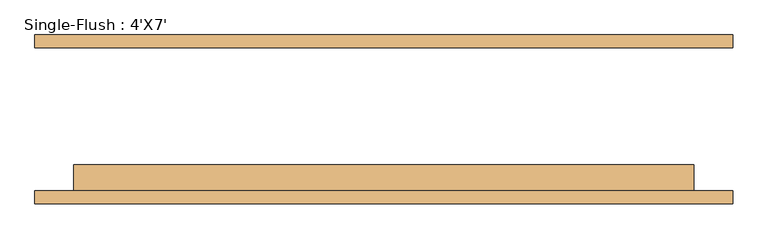
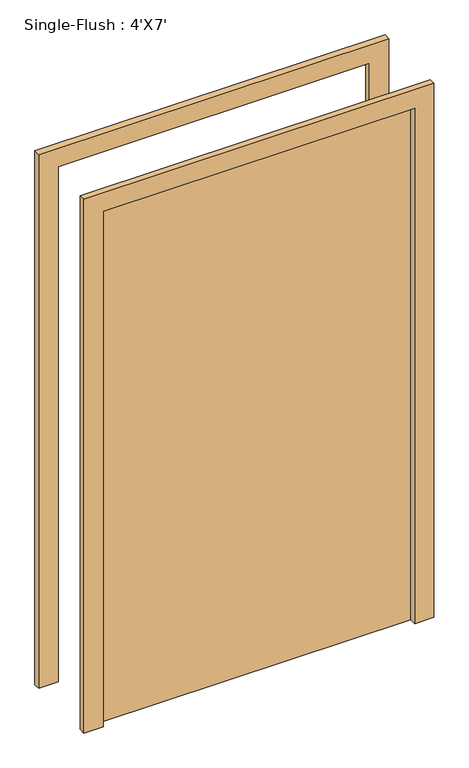
"""IFC4 building model written with IfcOpenShell, lengths in millimetres: door geometry, Single-Flush : 4'X7'."""

from ifc_helpers import new_model, si_unit, frame, origin, origin_with_axes, place, context, project, spatial, polyline, outline, extrude, source, transform, mapped, element, save


def single_flush_4_x7_d8936398(model_context):
    return source(origin(), model_context, "Body", "SweptSolid", [
        extrude(outline(polyline([(2209.8, -685.8), (0.0, -685.8), (0.0, -609.6), (2133.6, -609.6), (2133.6, 609.6), (0.0, 609.6), (0.0, 685.8), (2209.8, 685.8), (2209.8, -685.8)])), frame((0.0, -165.8, 0.0), z_axis=(0.0, 1.0, 0.0), x_axis=(0.0, 0.0, 1.0)), (0.0, 0.0, 1.0), 25.4),
        extrude(outline(polyline([(2209.8, 685.8), (2209.8, -685.8), (0.0, -685.8), (0.0, -609.6), (2133.6, -609.6), (2133.6, 609.6), (0.0, 609.6), (0.0, 685.8), (2209.8, 685.8)])), frame((0.0, 140.4, 0.0), z_axis=(0.0, 1.0, 0.0), x_axis=(0.0, 0.0, 1.0)), (0.0, 0.0, 1.0), 25.4),
        extrude(outline(polyline([(609.6, -89.6), (609.6, -140.4), (-609.6, -140.4), (-609.6, -89.6), (609.6, -89.6)])), origin_with_axes(), (0.0, 0.0, 1.0), 2133.6),
    ])


if __name__ == "__main__":
    model = new_model("IFC4")
    model_context = context("Model", 3, world=origin())
    ifc_project = project(units=[si_unit("LENGTHUNIT", "METRE", prefix="MILLI")], contexts=[model_context])
    site = spatial("IfcSite", under=ifc_project)
    building = spatial("IfcBuilding", under=site)
    placement = place(None, origin())
    single_flush_4_x7_shape = single_flush_4_x7_d8936398(model_context)
    element("IfcDoor", 1, ObjectType="Single-Flush : 4'X7'", at=placement, inside=building, context=model_context, shape_type="MappedRepresentation", body=[
        mapped(single_flush_4_x7_shape, transform((0.0, 0.0, 0.0), x_axis=(1.0, 0.0, 0.0), y_axis=(0.0, 1.0, 0.0), z_axis=(0.0, 0.0, 1.0))),
    ])
    save(model, "model.ifc")

# Revit data of these elements
# Type "Single-Flush : 4'X7'"
#   Type Mark = "11"
#   Assembly Code = "C1020"
#   Thickness = 0' - 2"
#   Height = 7' - 0"
#   Trim Projection Ext = 0' - 1"
#   Trim Projection Int = 0' - 1"
#   Trim Width = 0' - 3"
#   Width = 4' - 0"
#   Door Material = Door - Panel
#   Frame Material = Door - Frame
#   Function = (empty or 0)
#   Wall Closure = (empty or 0)
# Element 1 (IfcDoor, "Single-Flush : 4'X7'")
#   Materials on its faces: "Door - Frame", "Door - Panel"
# Materials
#   "Door - Panel": class "Wood", colour RGB 114 82 51, transparency 0
#   "Door - Frame": colour RGB 153 76 43, transparency 0
